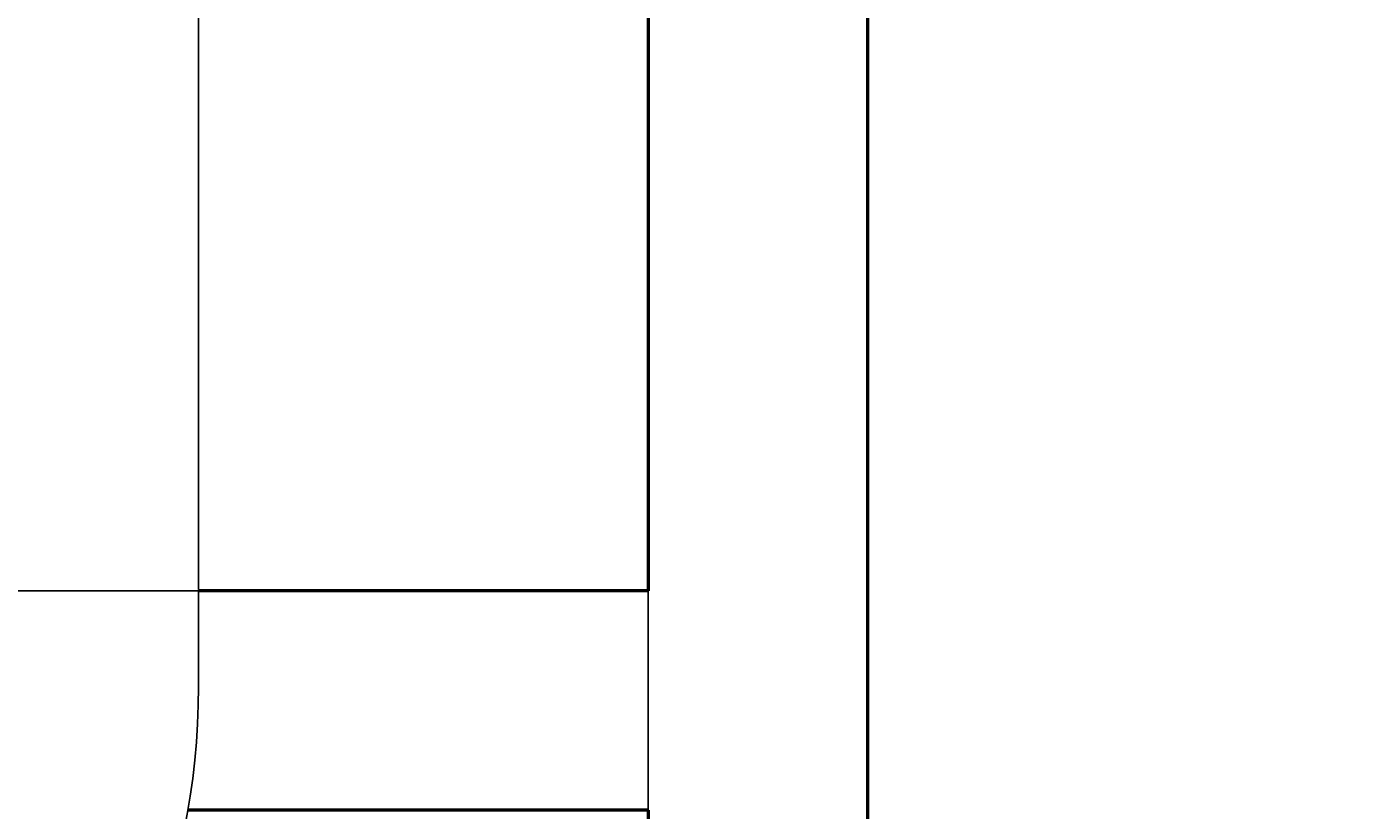
# Model space of a CAD drawing. Units: inches. Extents: x 37 to 824, y -700 to 234.
# Tile 71 of 77: x 394 to 449, y 75 to 107. Entities that reach past the tile are written whole.
import ezdxf

# ---------------------------------------------------------------- set-up
doc = ezdxf.new("R2010")
doc.units = ezdxf.units.IN
doc.header["$MEASUREMENT"] = 0
for name, color, linetype, lineweight in [('A-ANNO-DIMS', 2, 'Continuous', 18), ('A-DOOR', 4, 'Continuous', 25), ('A-WALL', 2, 'Continuous', 50)]:
    doc.layers.add(name, color=color, linetype=linetype, lineweight=lineweight)
doc.styles.get("Standard").update_dxf_attribs({"font": 'arial.ttf'})
doc.dimstyles.get("Standard").update_dxf_attribs({"dimtxt": 0.18, "dimasz": 0.18, "dimexe": 0.18, "dimexo": 0.0625, "dimgap": 0.09, "dimtad": 0, "dimtih": 1, "dimtoh": 1, "dimdec": 1, "dimzin": 0, "dimdsep": 46, "dimlunit": 4, "dimtxsty": 'Standard', "dimcen": 0.09, "dimadec": 0, "dimazin": 0, "dimtfac": 1, "dimtdec": 1, "dimtofl": 0, "dimtmove": 0, "dimatfit": 3, "dimfxl": 1, "dimtolj": 1, "dimtzin": 0, "dimarcsym": 0})

# ---------------------------------------------------------------- blocks, each defined once
blk = doc.blocks.new('*U6')
for p, q in [((-750, 0), (-750, -100)), ((0, 0), (0, -100))]:
    blk.add_line(p, q)
blk.add_lwpolyline([(0, 0), (0, 750), (-43.75, 750), (-43.75, 0)], close=True)
blk.add_arc((0, 0), 750, 90, 180)
blk = doc.blocks.new('*D60')
at = {"layer": 'A-ANNO-DIMS', "color": 0, "lineweight": -2, "ltscale": 0.5, "transparency": 16777216}
for p, q in [((419.015, 113.09), (78.159, 113.09)), ((78.339, 112.91), (78.339, 98.772)), ((78.339, 84.27), (78.339, 98.409)), ((419.015, 84.09), (78.159, 84.09))]:
    blk.add_line(p, q, dxfattribs=at)
at = {"layer": 'A-ANNO-DIMS', "color": 0, "ltscale": 0.5, "transparency": 16777216}
for points in [[(78.309, 112.91), (78.369, 112.91), (78.339, 113.09)], [(78.309, 84.27), (78.369, 84.27), (78.339, 84.09)]]:
    blk.add_solid(points, dxfattribs=at)
at = {"layer": 'Defpoints', "color": 0, "ltscale": 0.5, "transparency": 16777216}
for p in [(78.339, 113.09), (419.077, 113.09), (419.077, 84.09)]:
    blk.add_point(p, dxfattribs=at)
at = {"layer": 'A-ANNO-DIMS', "color": 0, "ltscale": 0.5, "transparency": 16777216, "insert": (78.339, 98.59), "char_height": 0.18, "attachment_point": 5}
blk.add_mtext('\\A1;2\'-5"', dxfattribs=at)
blk = doc.blocks.new('*D64')
at = {"layer": 'A-ANNO-DIMS', "color": 0, "lineweight": -2, "ltscale": 0.5, "transparency": 16777216}
for p, q in [((428.14, 191.09), (513.773, 191.09)), ((513.593, 190.91), (513.593, -87.228)), ((513.593, -365.73), (513.593, -87.591)), ((428.14, -365.91), (513.773, -365.91))]:
    blk.add_line(p, q, dxfattribs=at)
at = {"layer": 'A-ANNO-DIMS', "color": 0, "ltscale": 0.5, "transparency": 16777216}
for points in [[(513.563, 190.91), (513.623, 190.91), (513.593, 191.09)], [(513.563, -365.73), (513.623, -365.73), (513.593, -365.91)]]:
    blk.add_solid(points, dxfattribs=at)
at = {"layer": 'Defpoints', "color": 0, "ltscale": 0.5, "transparency": 16777216}
for p in [(428.077, 191.09), (428.077, -365.91), (513.593, -365.91)]:
    blk.add_point(p, dxfattribs=at)
at = {"layer": 'A-ANNO-DIMS', "color": 0, "ltscale": 0.5, "transparency": 16777216, "insert": (513.593, -87.41), "char_height": 0.18, "attachment_point": 5}
blk.add_mtext('\\A1;46\'-5"', dxfattribs=at)
blk = doc.blocks.new('*D74')
at = {"layer": 'A-ANNO-DIMS', "color": 0, "lineweight": -2, "ltscale": 0.5, "transparency": 16777216}
for p, q in [((371.077, 84.153), (371.077, 234.17)), ((371.257, 233.99), (385.3, 233.99)), ((400.425, 233.99), (386.381, 233.99)), ((400.605, 84.153), (400.605, 234.17))]:
    blk.add_line(p, q, dxfattribs=at)
at = {"layer": 'A-ANNO-DIMS', "color": 0, "ltscale": 0.5, "transparency": 16777216}
for points in [[(371.257, 234.02), (371.257, 233.96), (371.077, 233.99)], [(400.425, 234.02), (400.425, 233.96), (400.605, 233.99)]]:
    blk.add_solid(points, dxfattribs=at)
at = {"layer": 'Defpoints', "color": 0, "ltscale": 0.5, "transparency": 16777216}
for p in [(400.605, 233.99), (371.077, 84.09), (400.605, 84.09)]:
    blk.add_point(p, dxfattribs=at)
at = {"layer": 'A-ANNO-DIMS', "color": 0, "ltscale": 0.5, "transparency": 16777216, "insert": (385.841, 233.99), "char_height": 0.18, "attachment_point": 5}
blk.add_mtext('\\A1;2\'-5 1/2"', dxfattribs=at)
blk = doc.blocks.new('*D75')
at = {"layer": 'A-ANNO-DIMS', "color": 0, "lineweight": -2, "ltscale": 0.5, "transparency": 16777216}
for p, q in [((400.605, 84.153), (400.605, 234.17)), ((400.785, 233.99), (409.31, 233.99)), ((418.897, 233.99), (410.371, 233.99)), ((419.077, 84.153), (419.077, 234.17))]:
    blk.add_line(p, q, dxfattribs=at)
at = {"layer": 'A-ANNO-DIMS', "color": 0, "ltscale": 0.5, "transparency": 16777216}
for points in [[(400.785, 234.02), (400.785, 233.96), (400.605, 233.99)], [(418.897, 234.02), (418.897, 233.96), (419.077, 233.99)]]:
    blk.add_solid(points, dxfattribs=at)
at = {"layer": 'Defpoints', "color": 0, "ltscale": 0.5, "transparency": 16777216}
for p in [(419.077, 233.99), (400.605, 84.09), (419.077, 84.09)]:
    blk.add_point(p, dxfattribs=at)
at = {"layer": 'A-ANNO-DIMS', "color": 0, "ltscale": 0.5, "transparency": 16777216, "insert": (409.841, 233.99), "char_height": 0.18, "attachment_point": 5}
blk.add_mtext('\\A1;1\'-6 1/2"', dxfattribs=at)
blk = doc.blocks.new('*D83')
at = {"layer": 'A-ANNO-DIMS', "color": 0, "lineweight": -2, "ltscale": 0.5, "transparency": 16777216}
for p, q in [((358.132, -206.847), (358.132, 234.17)), ((358.312, 233.99), (388.275, 233.99)), ((418.897, 233.99), (388.934, 233.99)), ((419.077, -206.847), (419.077, 234.17))]:
    blk.add_line(p, q, dxfattribs=at)
at = {"layer": 'A-ANNO-DIMS', "color": 0, "ltscale": 0.5, "transparency": 16777216}
for points in [[(358.312, 234.02), (358.312, 233.96), (358.132, 233.99)], [(418.897, 234.02), (418.897, 233.96), (419.077, 233.99)]]:
    blk.add_solid(points, dxfattribs=at)
at = {"layer": 'Defpoints', "color": 0, "ltscale": 0.5, "transparency": 16777216}
for p in [(419.077, 233.99), (358.132, -206.91), (419.077, -206.91)]:
    blk.add_point(p, dxfattribs=at)
at = {"layer": 'A-ANNO-DIMS', "color": 0, "ltscale": 0.5, "transparency": 16777216, "insert": (388.605, 233.99), "char_height": 0.18, "attachment_point": 5}
blk.add_mtext('\\A1;5\'-1"', dxfattribs=at)

msp = doc.modelspace()

# ---------------------------------------------------------------- linework, layer by layer
at = {"layer": 'A-WALL'}
for p, q in [((428.077, 191.09), (428.077, 75.09)), ((419.077, 182.09), (419.077, 84.09)), ((419.077, 84.09), (400.605, 84.09)), ((419.077, 75.09), (400.167, 75.09)), ((419.077, 75.09), (419.077, 15.09)), ((428.077, 75.09), (428.077, 6.09))]:
    msp.add_line(p, q, dxfattribs=at)

# ---------------------------------------------------------------- block references
at = {"layer": 'A-DOOR', "xscale": 0.0393700787401575, "yscale": 0.0393700787401575, "zscale": 0.0393700787401575, "rotation": 180}
msp.add_blockref('*U6', (371.077, 80.153), dxfattribs=at)

# ---------------------------------------------------------------- dimensions: what is measured, and where the dimension line sits
at = {"layer": 'A-ANNO-DIMS', "ltscale": 0.5}
for base, p1, p2, picture, middle in [((419.077, 233.99), (358.132, -206.91), (419.077, -206.91), '*D83', (388.605, 233.99)), ((400.605, 233.99), (371.077, 84.09), (400.605, 84.09), '*D74', (385.841, 233.99)), ((419.077, 233.99), (400.605, 84.09), (419.077, 84.09), '*D75', (409.841, 233.99))]:
    dim = msp.add_linear_dim(base=base, p1=p1, p2=p2, dimstyle='Standard', override={"dimdec": 1, "dimlfac": 1, "dimrnd": 0, "dimzin": 1, "dimdsep": 46, "dimlunit": 4, "dimfrac": 2}, dxfattribs=at)
    dim.commit()
    dim.dimension.update_dxf_attribs({"geometry": picture, "text_midpoint": middle})
for base, p1, p2, picture, middle in [((513.593, -365.91), (428.077, 191.09), (428.077, -365.91), '*D64', (513.593, -87.41)), ((78.339, 113.09), (419.077, 84.09), (419.077, 113.09), '*D60', (78.339, 98.59))]:
    dim = msp.add_linear_dim(base=base, p1=p1, p2=p2, angle=90, dimstyle='Standard', override={"dimdec": 1, "dimlfac": 1, "dimrnd": 0, "dimzin": 1, "dimdsep": 46, "dimlunit": 4, "dimfrac": 2}, dxfattribs=at)
    dim.commit()
    dim.dimension.update_dxf_attribs({"geometry": picture, "text_midpoint": middle})

doc.saveas('drawing.dxf')
